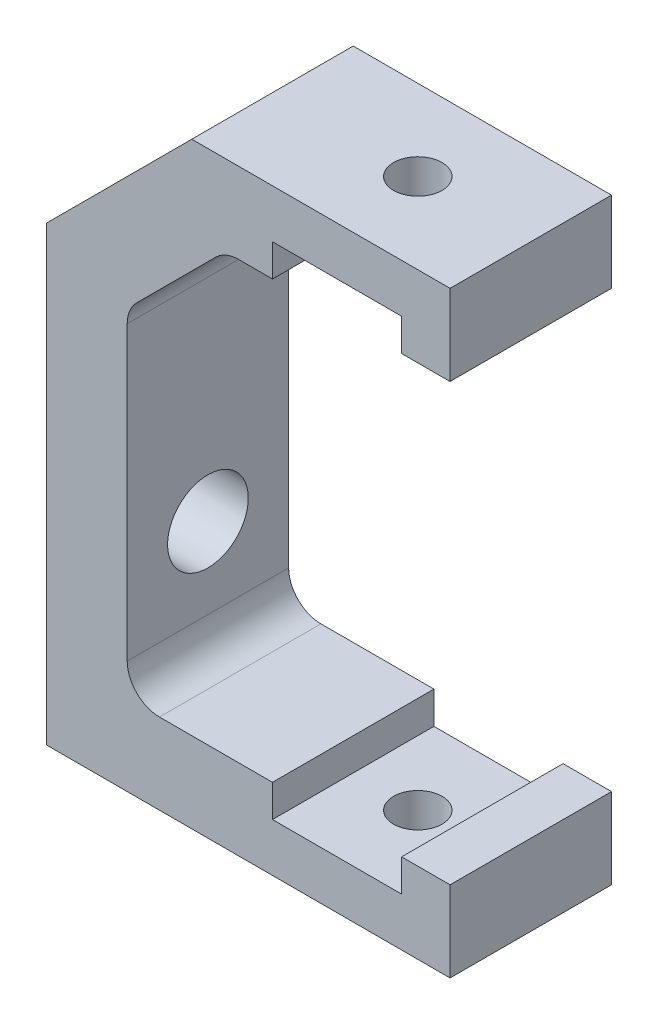
ISO-10303-21;
HEADER;
FILE_DESCRIPTION(('STEP AP214'),'2;1');
FILE_NAME('part.step','',(''),(''),'','','');
FILE_SCHEMA(('AUTOMOTIVE_DESIGN { 1 0 10303 214 1 1 1 1 }'));
ENDSEC;
DATA;
#1=APPLICATION_CONTEXT('core data for automotive mechanical design processes');
#2=APPLICATION_PROTOCOL_DEFINITION('international standard','automotive_design',2000,#1);
#3=PRODUCT_CONTEXT('',#1,'mechanical');
#4=PRODUCT('Part','Part','',(#3));
#5=PRODUCT_RELATED_PRODUCT_CATEGORY('part','',(#4));
#6=PRODUCT_DEFINITION_FORMATION('','',#4);
#7=PRODUCT_DEFINITION_CONTEXT('part definition',#1,'design');
#8=PRODUCT_DEFINITION('design','',#6,#7);
#9=PRODUCT_DEFINITION_SHAPE('','',#8);
#10=(LENGTH_UNIT() NAMED_UNIT(*) SI_UNIT(.MILLI.,.METRE.));
#11=(NAMED_UNIT(*) PLANE_ANGLE_UNIT() SI_UNIT($,.RADIAN.));
#12=(NAMED_UNIT(*) SI_UNIT($,.STERADIAN.) SOLID_ANGLE_UNIT());
#13=UNCERTAINTY_MEASURE_WITH_UNIT(LENGTH_MEASURE(1.E-05),#10,'distance_accuracy_value','');
#14=(GEOMETRIC_REPRESENTATION_CONTEXT(3) GLOBAL_UNCERTAINTY_ASSIGNED_CONTEXT((#13)) GLOBAL_UNIT_ASSIGNED_CONTEXT((#10,
#11,#12)) REPRESENTATION_CONTEXT('',''));
#15=CARTESIAN_POINT('',(0.,0.,0.));
#16=DIRECTION('',(0.,0.,1.));
#17=DIRECTION('',(1.,0.,0.));
#18=AXIS2_PLACEMENT_3D('',#15,#16,#17);
#19=CARTESIAN_POINT('',(0.,0.,10.));
#20=DIRECTION('',(0.,1.,0.));
#21=DIRECTION('',(0.,0.,1.));
#22=AXIS2_PLACEMENT_3D('',#19,#20,#21);
#23=PLANE('',#22);
#24=CARTESIAN_POINT('',(18.,0.,5.));
#25=DIRECTION('',(0.,1.,0.));
#26=DIRECTION('',(0.,0.,1.));
#27=AXIS2_PLACEMENT_3D('',#24,#25,#26);
#28=CIRCLE('',#27,1.5);
#29=CARTESIAN_POINT('',(18.,0.,6.5));
#30=VERTEX_POINT('',#29);
#31=EDGE_CURVE('E222',#30,#30,#28,.T.);
#32=ORIENTED_EDGE('',*,*,#31,.T.);
#33=EDGE_LOOP('',(#32));
#34=FACE_BOUND('',#33,.T.);
#35=DIRECTION('',(1.,0.,0.));
#36=VECTOR('',#35,1.);
#37=CARTESIAN_POINT('',(0.,0.,0.));
#38=LINE('',#37,#36);
#39=CARTESIAN_POINT('',(0.,0.,0.));
#40=VERTEX_POINT('',#39);
#41=CARTESIAN_POINT('',(25.,0.,0.));
#42=VERTEX_POINT('',#41);
#43=EDGE_CURVE('E220',#40,#42,#38,.T.);
#44=ORIENTED_EDGE('',*,*,#43,.T.);
#45=DIRECTION('',(0.,0.,-1.));
#46=VECTOR('',#45,1.);
#47=CARTESIAN_POINT('',(25.,0.,10.));
#48=LINE('',#47,#46);
#49=CARTESIAN_POINT('',(25.,0.,10.));
#50=VERTEX_POINT('',#49);
#51=EDGE_CURVE('E11',#50,#42,#48,.T.);
#52=ORIENTED_EDGE('',*,*,#51,.F.);
#53=DIRECTION('',(1.,0.,0.));
#54=VECTOR('',#53,1.);
#55=CARTESIAN_POINT('',(0.,0.,10.));
#56=LINE('',#55,#54);
#57=CARTESIAN_POINT('',(0.,0.,10.));
#58=VERTEX_POINT('',#57);
#59=EDGE_CURVE('E256',#58,#50,#56,.T.);
#60=ORIENTED_EDGE('',*,*,#59,.F.);
#61=DIRECTION('',(0.,0.,-1.));
#62=VECTOR('',#61,1.);
#63=CARTESIAN_POINT('',(0.,0.,10.));
#64=LINE('',#63,#62);
#65=EDGE_CURVE('E213',#58,#40,#64,.T.);
#66=ORIENTED_EDGE('',*,*,#65,.T.);
#67=EDGE_LOOP('',(#44,#52,#60,#66));
#68=FACE_BOUND('',#67,.T.);
#69=ADVANCED_FACE('F43',(#34,#68),#23,.F.);
#70=CARTESIAN_POINT('',(25.,0.,10.));
#71=DIRECTION('',(-1.,0.,0.));
#72=DIRECTION('',(0.,0.,1.));
#73=AXIS2_PLACEMENT_3D('',#70,#71,#72);
#74=PLANE('',#73);
#75=DIRECTION('',(0.,1.,0.));
#76=VECTOR('',#75,1.);
#77=CARTESIAN_POINT('',(25.,0.,0.));
#78=LINE('',#77,#76);
#79=CARTESIAN_POINT('',(25.,5.,0.));
#80=VERTEX_POINT('',#79);
#81=EDGE_CURVE('E219',#42,#80,#78,.T.);
#82=ORIENTED_EDGE('',*,*,#81,.T.);
#83=DIRECTION('',(0.,0.,-1.));
#84=VECTOR('',#83,1.);
#85=CARTESIAN_POINT('',(25.,5.,10.));
#86=LINE('',#85,#84);
#87=CARTESIAN_POINT('',(25.,5.,10.));
#88=VERTEX_POINT('',#87);
#89=EDGE_CURVE('E51',#88,#80,#86,.T.);
#90=ORIENTED_EDGE('',*,*,#89,.F.);
#91=DIRECTION('',(0.,1.,0.));
#92=VECTOR('',#91,1.);
#93=CARTESIAN_POINT('',(25.,0.,10.));
#94=LINE('',#93,#92);
#95=EDGE_CURVE('E143',#50,#88,#94,.T.);
#96=ORIENTED_EDGE('',*,*,#95,.F.);
#97=ORIENTED_EDGE('',*,*,#51,.T.);
#98=EDGE_LOOP('',(#82,#90,#96,#97));
#99=FACE_BOUND('',#98,.T.);
#100=ADVANCED_FACE('F382',(#99),#74,.F.);
#101=CARTESIAN_POINT('',(25.,5.,10.));
#102=DIRECTION('',(0.,-1.,0.));
#103=DIRECTION('',(0.,0.,-1.));
#104=AXIS2_PLACEMENT_3D('',#101,#102,#103);
#105=PLANE('',#104);
#106=DIRECTION('',(-1.,0.,0.));
#107=VECTOR('',#106,1.);
#108=CARTESIAN_POINT('',(25.,5.,0.));
#109=LINE('',#108,#107);
#110=CARTESIAN_POINT('',(22.,5.,0.));
#111=VERTEX_POINT('',#110);
#112=EDGE_CURVE('E224',#80,#111,#109,.T.);
#113=ORIENTED_EDGE('',*,*,#112,.T.);
#114=DIRECTION('',(0.,0.,-1.));
#115=VECTOR('',#114,1.);
#116=CARTESIAN_POINT('',(22.,5.,10.));
#117=LINE('',#116,#115);
#118=CARTESIAN_POINT('',(22.,5.,10.));
#119=VERTEX_POINT('',#118);
#120=EDGE_CURVE('E301',#119,#111,#117,.T.);
#121=ORIENTED_EDGE('',*,*,#120,.F.);
#122=DIRECTION('',(-1.,0.,0.));
#123=VECTOR('',#122,1.);
#124=CARTESIAN_POINT('',(25.,5.,10.));
#125=LINE('',#124,#123);
#126=EDGE_CURVE('E315',#88,#119,#125,.T.);
#127=ORIENTED_EDGE('',*,*,#126,.F.);
#128=ORIENTED_EDGE('',*,*,#89,.T.);
#129=EDGE_LOOP('',(#113,#121,#127,#128));
#130=FACE_BOUND('',#129,.T.);
#131=ADVANCED_FACE('F309',(#130),#105,.F.);
#132=CARTESIAN_POINT('',(22.,5.,10.));
#133=DIRECTION('',(1.,0.,0.));
#134=DIRECTION('',(0.,0.,-1.));
#135=AXIS2_PLACEMENT_3D('',#132,#133,#134);
#136=PLANE('',#135);
#137=DIRECTION('',(0.,-1.,0.));
#138=VECTOR('',#137,1.);
#139=CARTESIAN_POINT('',(22.,5.,0.));
#140=LINE('',#139,#138);
#141=CARTESIAN_POINT('',(22.,3.,0.));
#142=VERTEX_POINT('',#141);
#143=EDGE_CURVE('E223',#111,#142,#140,.T.);
#144=ORIENTED_EDGE('',*,*,#143,.T.);
#145=DIRECTION('',(0.,0.,-1.));
#146=VECTOR('',#145,1.);
#147=CARTESIAN_POINT('',(22.,3.,10.));
#148=LINE('',#147,#146);
#149=CARTESIAN_POINT('',(22.,3.,10.));
#150=VERTEX_POINT('',#149);
#151=EDGE_CURVE('E302',#150,#142,#148,.T.);
#152=ORIENTED_EDGE('',*,*,#151,.F.);
#153=DIRECTION('',(0.,-1.,0.));
#154=VECTOR('',#153,1.);
#155=CARTESIAN_POINT('',(22.,5.,10.));
#156=LINE('',#155,#154);
#157=EDGE_CURVE('E329',#119,#150,#156,.T.);
#158=ORIENTED_EDGE('',*,*,#157,.F.);
#159=ORIENTED_EDGE('',*,*,#120,.T.);
#160=EDGE_LOOP('',(#144,#152,#158,#159));
#161=FACE_BOUND('',#160,.T.);
#162=ADVANCED_FACE('F321',(#161),#136,.F.);
#163=CARTESIAN_POINT('',(22.,3.,10.));
#164=DIRECTION('',(0.,-1.,0.));
#165=DIRECTION('',(0.,0.,-1.));
#166=AXIS2_PLACEMENT_3D('',#163,#164,#165);
#167=PLANE('',#166);
#168=CARTESIAN_POINT('',(18.,3.,5.));
#169=DIRECTION('',(0.,1.,0.));
#170=DIRECTION('',(0.,0.,1.));
#171=AXIS2_PLACEMENT_3D('',#168,#169,#170);
#172=CIRCLE('',#171,1.5);
#173=CARTESIAN_POINT('',(18.,3.,6.5));
#174=VERTEX_POINT('',#173);
#175=EDGE_CURVE('E391',#174,#174,#172,.T.);
#176=ORIENTED_EDGE('',*,*,#175,.F.);
#177=EDGE_LOOP('',(#176));
#178=FACE_BOUND('',#177,.T.);
#179=DIRECTION('',(-1.,0.,0.));
#180=VECTOR('',#179,1.);
#181=CARTESIAN_POINT('',(22.,3.,0.));
#182=LINE('',#181,#180);
#183=CARTESIAN_POINT('',(14.,3.,0.));
#184=VERTEX_POINT('',#183);
#185=EDGE_CURVE('E227',#142,#184,#182,.T.);
#186=ORIENTED_EDGE('',*,*,#185,.T.);
#187=DIRECTION('',(0.,0.,-1.));
#188=VECTOR('',#187,1.);
#189=CARTESIAN_POINT('',(14.,3.,10.));
#190=LINE('',#189,#188);
#191=CARTESIAN_POINT('',(14.,3.,10.));
#192=VERTEX_POINT('',#191);
#193=EDGE_CURVE('E299',#192,#184,#190,.T.);
#194=ORIENTED_EDGE('',*,*,#193,.F.);
#195=DIRECTION('',(-1.,0.,0.));
#196=VECTOR('',#195,1.);
#197=CARTESIAN_POINT('',(22.,3.,10.));
#198=LINE('',#197,#196);
#199=EDGE_CURVE('E330',#150,#192,#198,.T.);
#200=ORIENTED_EDGE('',*,*,#199,.F.);
#201=ORIENTED_EDGE('',*,*,#151,.T.);
#202=EDGE_LOOP('',(#186,#194,#200,#201));
#203=FACE_BOUND('',#202,.T.);
#204=ADVANCED_FACE('F324',(#178,#203),#167,.F.);
#205=CARTESIAN_POINT('',(14.,3.,10.));
#206=DIRECTION('',(-1.,0.,0.));
#207=DIRECTION('',(0.,0.,1.));
#208=AXIS2_PLACEMENT_3D('',#205,#206,#207);
#209=PLANE('',#208);
#210=DIRECTION('',(0.,1.,0.));
#211=VECTOR('',#210,1.);
#212=CARTESIAN_POINT('',(14.,3.,0.));
#213=LINE('',#212,#211);
#214=CARTESIAN_POINT('',(14.,5.,0.));
#215=VERTEX_POINT('',#214);
#216=EDGE_CURVE('E228',#184,#215,#213,.T.);
#217=ORIENTED_EDGE('',*,*,#216,.T.);
#218=DIRECTION('',(0.,0.,-1.));
#219=VECTOR('',#218,1.);
#220=CARTESIAN_POINT('',(14.,5.,10.));
#221=LINE('',#220,#219);
#222=CARTESIAN_POINT('',(14.,5.,10.));
#223=VERTEX_POINT('',#222);
#224=EDGE_CURVE('E293',#223,#215,#221,.T.);
#225=ORIENTED_EDGE('',*,*,#224,.F.);
#226=DIRECTION('',(0.,1.,0.));
#227=VECTOR('',#226,1.);
#228=CARTESIAN_POINT('',(14.,3.,10.));
#229=LINE('',#228,#227);
#230=EDGE_CURVE('E328',#192,#223,#229,.T.);
#231=ORIENTED_EDGE('',*,*,#230,.F.);
#232=ORIENTED_EDGE('',*,*,#193,.T.);
#233=EDGE_LOOP('',(#217,#225,#231,#232));
#234=FACE_BOUND('',#233,.T.);
#235=ADVANCED_FACE('F451',(#234),#209,.F.);
#236=CARTESIAN_POINT('',(7.00000000000002,5.,10.));
#237=DIRECTION('',(0.,-1.,0.));
#238=DIRECTION('',(0.,0.,-1.));
#239=AXIS2_PLACEMENT_3D('',#236,#237,#238);
#240=PLANE('',#239);
#241=DIRECTION('',(-1.,0.,0.));
#242=VECTOR('',#241,1.);
#243=CARTESIAN_POINT('',(7.00000000000002,5.,0.));
#244=LINE('',#243,#242);
#245=CARTESIAN_POINT('',(7.00000000000002,5.,0.));
#246=VERTEX_POINT('',#245);
#247=EDGE_CURVE('E232',#215,#246,#244,.T.);
#248=ORIENTED_EDGE('',*,*,#247,.T.);
#249=DIRECTION('',(0.,0.,-1.));
#250=VECTOR('',#249,1.);
#251=CARTESIAN_POINT('',(7.00000000000002,5.,10.));
#252=LINE('',#251,#250);
#253=CARTESIAN_POINT('',(7.00000000000002,5.,10.));
#254=VERTEX_POINT('',#253);
#255=EDGE_CURVE('E295',#254,#246,#252,.T.);
#256=ORIENTED_EDGE('',*,*,#255,.F.);
#257=DIRECTION('',(-1.,0.,0.));
#258=VECTOR('',#257,1.);
#259=CARTESIAN_POINT('',(7.00000000000002,5.,10.));
#260=LINE('',#259,#258);
#261=EDGE_CURVE('E335',#223,#254,#260,.T.);
#262=ORIENTED_EDGE('',*,*,#261,.F.);
#263=ORIENTED_EDGE('',*,*,#224,.T.);
#264=EDGE_LOOP('',(#248,#256,#262,#263));
#265=FACE_BOUND('',#264,.T.);
#266=ADVANCED_FACE('F452',(#265),#240,.F.);
#267=CARTESIAN_POINT('',(7.,7.,10.));
#268=DIRECTION('',(0.,0.,-1.));
#269=DIRECTION('',(-1.,0.,0.));
#270=AXIS2_PLACEMENT_3D('',#267,#268,#269);
#271=CYLINDRICAL_SURFACE('',#270,2.);
#272=CARTESIAN_POINT('',(7.,7.,0.));
#273=DIRECTION('',(0.,0.,-1.));
#274=DIRECTION('',(-1.,0.,0.));
#275=AXIS2_PLACEMENT_3D('',#272,#273,#274);
#276=CIRCLE('',#275,2.);
#277=CARTESIAN_POINT('',(5.,7.00000000000002,0.));
#278=VERTEX_POINT('',#277);
#279=EDGE_CURVE('E234',#246,#278,#276,.T.);
#280=ORIENTED_EDGE('',*,*,#279,.T.);
#281=DIRECTION('',(0.,0.,-1.));
#282=VECTOR('',#281,1.);
#283=CARTESIAN_POINT('',(5.,7.00000000000002,10.));
#284=LINE('',#283,#282);
#285=CARTESIAN_POINT('',(5.,7.00000000000002,10.));
#286=VERTEX_POINT('',#285);
#287=EDGE_CURVE('E286',#286,#278,#284,.T.);
#288=ORIENTED_EDGE('',*,*,#287,.F.);
#289=CARTESIAN_POINT('',(7.,7.,10.));
#290=DIRECTION('',(0.,0.,-1.));
#291=DIRECTION('',(-1.,0.,0.));
#292=AXIS2_PLACEMENT_3D('',#289,#290,#291);
#293=CIRCLE('',#292,2.);
#294=EDGE_CURVE('E339',#254,#286,#293,.T.);
#295=ORIENTED_EDGE('',*,*,#294,.F.);
#296=ORIENTED_EDGE('',*,*,#255,.T.);
#297=EDGE_LOOP('',(#280,#288,#295,#296));
#298=FACE_BOUND('',#297,.T.);
#299=ADVANCED_FACE('F423',(#298),#271,.F.);
#300=CARTESIAN_POINT('',(5.,25.1005050633883,10.));
#301=DIRECTION('',(-1.,0.,0.));
#302=DIRECTION('',(0.,-1.,0.));
#303=AXIS2_PLACEMENT_3D('',#300,#301,#302);
#304=PLANE('',#303);
#305=CARTESIAN_POINT('',(5.,12.,5.));
#306=DIRECTION('',(-1.,0.,0.));
#307=DIRECTION('',(0.,-1.,0.));
#308=AXIS2_PLACEMENT_3D('',#305,#306,#307);
#309=CIRCLE('',#308,2.5);
#310=CARTESIAN_POINT('',(5.,9.5,5.));
#311=VERTEX_POINT('',#310);
#312=EDGE_CURVE('E404',#311,#311,#309,.T.);
#313=ORIENTED_EDGE('',*,*,#312,.T.);
#314=EDGE_LOOP('',(#313));
#315=FACE_BOUND('',#314,.T.);
#316=DIRECTION('',(0.,1.,0.));
#317=VECTOR('',#316,1.);
#318=CARTESIAN_POINT('',(5.,25.1005050633883,0.));
#319=LINE('',#318,#317);
#320=CARTESIAN_POINT('',(5.,25.1005050633883,0.));
#321=VERTEX_POINT('',#320);
#322=EDGE_CURVE('E233',#278,#321,#319,.T.);
#323=ORIENTED_EDGE('',*,*,#322,.T.);
#324=DIRECTION('',(0.,0.,-1.));
#325=VECTOR('',#324,1.);
#326=CARTESIAN_POINT('',(5.,25.1005050633883,10.));
#327=LINE('',#326,#325);
#328=CARTESIAN_POINT('',(5.,25.1005050633883,10.));
#329=VERTEX_POINT('',#328);
#330=EDGE_CURVE('E287',#329,#321,#327,.T.);
#331=ORIENTED_EDGE('',*,*,#330,.F.);
#332=DIRECTION('',(0.,1.,0.));
#333=VECTOR('',#332,1.);
#334=CARTESIAN_POINT('',(5.,25.1005050633883,10.));
#335=LINE('',#334,#333);
#336=EDGE_CURVE('E340',#286,#329,#335,.T.);
#337=ORIENTED_EDGE('',*,*,#336,.F.);
#338=ORIENTED_EDGE('',*,*,#287,.T.);
#339=EDGE_LOOP('',(#323,#331,#337,#338));
#340=FACE_BOUND('',#339,.T.);
#341=ADVANCED_FACE('F417',(#315,#340),#304,.F.);
#342=CARTESIAN_POINT('',(7.,25.1005050633883,10.));
#343=DIRECTION('',(0.,0.,-1.));
#344=DIRECTION('',(-1.,0.,0.));
#345=AXIS2_PLACEMENT_3D('',#342,#343,#344);
#346=CYLINDRICAL_SURFACE('',#345,2.);
#347=CARTESIAN_POINT('',(7.,25.1005050633883,0.));
#348=DIRECTION('',(0.,0.,-1.));
#349=DIRECTION('',(1.,0.,0.));
#350=AXIS2_PLACEMENT_3D('',#347,#348,#349);
#351=CIRCLE('',#350,2.);
#352=CARTESIAN_POINT('',(5.5857864376269,26.5147186257614,0.));
#353=VERTEX_POINT('',#352);
#354=EDGE_CURVE('E240',#321,#353,#351,.T.);
#355=ORIENTED_EDGE('',*,*,#354,.T.);
#356=DIRECTION('',(0.,0.,-1.));
#357=VECTOR('',#356,1.);
#358=CARTESIAN_POINT('',(5.5857864376269,26.5147186257614,10.));
#359=LINE('',#358,#357);
#360=CARTESIAN_POINT('',(5.5857864376269,26.5147186257614,10.));
#361=VERTEX_POINT('',#360);
#362=EDGE_CURVE('E284',#361,#353,#359,.T.);
#363=ORIENTED_EDGE('',*,*,#362,.F.);
#364=CARTESIAN_POINT('',(7.,25.1005050633883,10.));
#365=DIRECTION('',(0.,0.,-1.));
#366=DIRECTION('',(1.,0.,0.));
#367=AXIS2_PLACEMENT_3D('',#364,#365,#366);
#368=CIRCLE('',#367,2.);
#369=EDGE_CURVE('E345',#329,#361,#368,.T.);
#370=ORIENTED_EDGE('',*,*,#369,.F.);
#371=ORIENTED_EDGE('',*,*,#330,.T.);
#372=EDGE_LOOP('',(#355,#363,#370,#371));
#373=FACE_BOUND('',#372,.T.);
#374=ADVANCED_FACE('F419',(#373),#346,.F.);
#375=CARTESIAN_POINT('',(5.5857864376269,26.5147186257614,10.));
#376=DIRECTION('',(-0.707106781186549,0.707106781186546,0.));
#377=DIRECTION('',(-0.707106781186546,-0.707106781186549,0.));
#378=AXIS2_PLACEMENT_3D('',#375,#376,#377);
#379=PLANE('',#378);
#380=DIRECTION('',(0.707106781186546,0.707106781186549,0.));
#381=VECTOR('',#380,1.);
#382=CARTESIAN_POINT('',(5.5857864376269,26.5147186257614,0.));
#383=LINE('',#382,#381);
#384=CARTESIAN_POINT('',(10.4852813742385,31.4142135623731,0.));
#385=VERTEX_POINT('',#384);
#386=EDGE_CURVE('E239',#353,#385,#383,.T.);
#387=ORIENTED_EDGE('',*,*,#386,.T.);
#388=DIRECTION('',(0.,0.,-1.));
#389=VECTOR('',#388,1.);
#390=CARTESIAN_POINT('',(10.4852813742385,31.4142135623731,10.));
#391=LINE('',#390,#389);
#392=CARTESIAN_POINT('',(10.4852813742385,31.4142135623731,10.));
#393=VERTEX_POINT('',#392);
#394=EDGE_CURVE('E278',#393,#385,#391,.T.);
#395=ORIENTED_EDGE('',*,*,#394,.F.);
#396=DIRECTION('',(0.707106781186546,0.707106781186549,0.));
#397=VECTOR('',#396,1.);
#398=CARTESIAN_POINT('',(5.5857864376269,26.5147186257614,10.));
#399=LINE('',#398,#397);
#400=EDGE_CURVE('E341',#361,#393,#399,.T.);
#401=ORIENTED_EDGE('',*,*,#400,.F.);
#402=ORIENTED_EDGE('',*,*,#362,.T.);
#403=EDGE_LOOP('',(#387,#395,#401,#402));
#404=FACE_BOUND('',#403,.T.);
#405=ADVANCED_FACE('F440',(#404),#379,.F.);
#406=CARTESIAN_POINT('',(11.8994949366116,30.,10.));
#407=DIRECTION('',(0.,0.,-1.));
#408=DIRECTION('',(-1.,0.,0.));
#409=AXIS2_PLACEMENT_3D('',#406,#407,#408);
#410=CYLINDRICAL_SURFACE('',#409,2.);
#411=CARTESIAN_POINT('',(11.8994949366116,30.,0.));
#412=DIRECTION('',(0.,0.,-1.));
#413=DIRECTION('',(1.,0.,0.));
#414=AXIS2_PLACEMENT_3D('',#411,#412,#413);
#415=CIRCLE('',#414,2.);
#416=CARTESIAN_POINT('',(11.8994949366116,32.,0.));
#417=VERTEX_POINT('',#416);
#418=EDGE_CURVE('E241',#385,#417,#415,.T.);
#419=ORIENTED_EDGE('',*,*,#418,.T.);
#420=DIRECTION('',(0.,0.,-1.));
#421=VECTOR('',#420,1.);
#422=CARTESIAN_POINT('',(11.8994949366116,32.,10.));
#423=LINE('',#422,#421);
#424=CARTESIAN_POINT('',(11.8994949366116,32.,10.));
#425=VERTEX_POINT('',#424);
#426=EDGE_CURVE('E280',#425,#417,#423,.T.);
#427=ORIENTED_EDGE('',*,*,#426,.F.);
#428=CARTESIAN_POINT('',(11.8994949366116,30.,10.));
#429=DIRECTION('',(0.,0.,-1.));
#430=DIRECTION('',(1.,0.,0.));
#431=AXIS2_PLACEMENT_3D('',#428,#429,#430);
#432=CIRCLE('',#431,2.);
#433=EDGE_CURVE('E347',#393,#425,#432,.T.);
#434=ORIENTED_EDGE('',*,*,#433,.F.);
#435=ORIENTED_EDGE('',*,*,#394,.T.);
#436=EDGE_LOOP('',(#419,#427,#434,#435));
#437=FACE_BOUND('',#436,.T.);
#438=ADVANCED_FACE('F442',(#437),#410,.F.);
#439=CARTESIAN_POINT('',(11.8994949366116,32.,10.));
#440=DIRECTION('',(0.,1.,0.));
#441=DIRECTION('',(0.,0.,1.));
#442=AXIS2_PLACEMENT_3D('',#439,#440,#441);
#443=PLANE('',#442);
#444=DIRECTION('',(1.,0.,0.));
#445=VECTOR('',#444,1.);
#446=CARTESIAN_POINT('',(11.8994949366116,32.,0.));
#447=LINE('',#446,#445);
#448=CARTESIAN_POINT('',(14.,32.,0.));
#449=VERTEX_POINT('',#448);
#450=EDGE_CURVE('E244',#417,#449,#447,.T.);
#451=ORIENTED_EDGE('',*,*,#450,.T.);
#452=DIRECTION('',(0.,0.,-1.));
#453=VECTOR('',#452,1.);
#454=CARTESIAN_POINT('',(14.,32.,10.));
#455=LINE('',#454,#453);
#456=CARTESIAN_POINT('',(14.,32.,10.));
#457=VERTEX_POINT('',#456);
#458=EDGE_CURVE('E273',#457,#449,#455,.T.);
#459=ORIENTED_EDGE('',*,*,#458,.F.);
#460=DIRECTION('',(1.,0.,0.));
#461=VECTOR('',#460,1.);
#462=CARTESIAN_POINT('',(11.8994949366116,32.,10.));
#463=LINE('',#462,#461);
#464=EDGE_CURVE('E346',#425,#457,#463,.T.);
#465=ORIENTED_EDGE('',*,*,#464,.F.);
#466=ORIENTED_EDGE('',*,*,#426,.T.);
#467=EDGE_LOOP('',(#451,#459,#465,#466));
#468=FACE_BOUND('',#467,.T.);
#469=ADVANCED_FACE('F531',(#468),#443,.F.);
#470=CARTESIAN_POINT('',(14.,34.,10.));
#471=DIRECTION('',(-1.,0.,0.));
#472=DIRECTION('',(0.,0.,1.));
#473=AXIS2_PLACEMENT_3D('',#470,#471,#472);
#474=PLANE('',#473);
#475=DIRECTION('',(0.,1.,0.));
#476=VECTOR('',#475,1.);
#477=CARTESIAN_POINT('',(14.,34.,0.));
#478=LINE('',#477,#476);
#479=CARTESIAN_POINT('',(14.,34.,0.));
#480=VERTEX_POINT('',#479);
#481=EDGE_CURVE('E245',#449,#480,#478,.T.);
#482=ORIENTED_EDGE('',*,*,#481,.T.);
#483=DIRECTION('',(0.,0.,-1.));
#484=VECTOR('',#483,1.);
#485=CARTESIAN_POINT('',(14.,34.,10.));
#486=LINE('',#485,#484);
#487=CARTESIAN_POINT('',(14.,34.,10.));
#488=VERTEX_POINT('',#487);
#489=EDGE_CURVE('E271',#488,#480,#486,.T.);
#490=ORIENTED_EDGE('',*,*,#489,.F.);
#491=DIRECTION('',(0.,1.,0.));
#492=VECTOR('',#491,1.);
#493=CARTESIAN_POINT('',(14.,34.,10.));
#494=LINE('',#493,#492);
#495=EDGE_CURVE('E348',#457,#488,#494,.T.);
#496=ORIENTED_EDGE('',*,*,#495,.F.);
#497=ORIENTED_EDGE('',*,*,#458,.T.);
#498=EDGE_LOOP('',(#482,#490,#496,#497));
#499=FACE_BOUND('',#498,.T.);
#500=ADVANCED_FACE('F545',(#499),#474,.F.);
#501=CARTESIAN_POINT('',(22.,34.,10.));
#502=DIRECTION('',(0.,1.,0.));
#503=DIRECTION('',(0.,0.,1.));
#504=AXIS2_PLACEMENT_3D('',#501,#502,#503);
#505=PLANE('',#504);
#506=CARTESIAN_POINT('',(18.,34.,5.));
#507=DIRECTION('',(0.,1.,0.));
#508=DIRECTION('',(0.,0.,1.));
#509=AXIS2_PLACEMENT_3D('',#506,#507,#508);
#510=CIRCLE('',#509,1.5);
#511=CARTESIAN_POINT('',(18.,34.,6.5));
#512=VERTEX_POINT('',#511);
#513=EDGE_CURVE('E393',#512,#512,#510,.T.);
#514=ORIENTED_EDGE('',*,*,#513,.T.);
#515=EDGE_LOOP('',(#514));
#516=FACE_BOUND('',#515,.T.);
#517=DIRECTION('',(1.,0.,0.));
#518=VECTOR('',#517,1.);
#519=CARTESIAN_POINT('',(22.,34.,0.));
#520=LINE('',#519,#518);
#521=CARTESIAN_POINT('',(22.,34.,0.));
#522=VERTEX_POINT('',#521);
#523=EDGE_CURVE('E250',#480,#522,#520,.T.);
#524=ORIENTED_EDGE('',*,*,#523,.T.);
#525=DIRECTION('',(0.,0.,-1.));
#526=VECTOR('',#525,1.);
#527=CARTESIAN_POINT('',(22.,34.,10.));
#528=LINE('',#527,#526);
#529=CARTESIAN_POINT('',(22.,34.,10.));
#530=VERTEX_POINT('',#529);
#531=EDGE_CURVE('E268',#530,#522,#528,.T.);
#532=ORIENTED_EDGE('',*,*,#531,.F.);
#533=DIRECTION('',(1.,0.,0.));
#534=VECTOR('',#533,1.);
#535=CARTESIAN_POINT('',(22.,34.,10.));
#536=LINE('',#535,#534);
#537=EDGE_CURVE('E352',#488,#530,#536,.T.);
#538=ORIENTED_EDGE('',*,*,#537,.F.);
#539=ORIENTED_EDGE('',*,*,#489,.T.);
#540=EDGE_LOOP('',(#524,#532,#538,#539));
#541=FACE_BOUND('',#540,.T.);
#542=ADVANCED_FACE('F555',(#516,#541),#505,.F.);
#543=CARTESIAN_POINT('',(22.,32.,10.));
#544=DIRECTION('',(1.,0.,0.));
#545=DIRECTION('',(0.,0.,-1.));
#546=AXIS2_PLACEMENT_3D('',#543,#544,#545);
#547=PLANE('',#546);
#548=DIRECTION('',(0.,-1.,0.));
#549=VECTOR('',#548,1.);
#550=CARTESIAN_POINT('',(22.,32.,0.));
#551=LINE('',#550,#549);
#552=CARTESIAN_POINT('',(22.,32.,0.));
#553=VERTEX_POINT('',#552);
#554=EDGE_CURVE('E246',#522,#553,#551,.T.);
#555=ORIENTED_EDGE('',*,*,#554,.T.);
#556=DIRECTION('',(0.,0.,-1.));
#557=VECTOR('',#556,1.);
#558=CARTESIAN_POINT('',(22.,32.,10.));
#559=LINE('',#558,#557);
#560=CARTESIAN_POINT('',(22.,32.,10.));
#561=VERTEX_POINT('',#560);
#562=EDGE_CURVE('E264',#561,#553,#559,.T.);
#563=ORIENTED_EDGE('',*,*,#562,.F.);
#564=DIRECTION('',(0.,-1.,0.));
#565=VECTOR('',#564,1.);
#566=CARTESIAN_POINT('',(22.,32.,10.));
#567=LINE('',#566,#565);
#568=EDGE_CURVE('E353',#530,#561,#567,.T.);
#569=ORIENTED_EDGE('',*,*,#568,.F.);
#570=ORIENTED_EDGE('',*,*,#531,.T.);
#571=EDGE_LOOP('',(#555,#563,#569,#570));
#572=FACE_BOUND('',#571,.T.);
#573=ADVANCED_FACE('F564',(#572),#547,.F.);
#574=CARTESIAN_POINT('',(25.,32.,10.));
#575=DIRECTION('',(0.,1.,0.));
#576=DIRECTION('',(0.,0.,1.));
#577=AXIS2_PLACEMENT_3D('',#574,#575,#576);
#578=PLANE('',#577);
#579=DIRECTION('',(1.,0.,0.));
#580=VECTOR('',#579,1.);
#581=CARTESIAN_POINT('',(25.,32.,0.));
#582=LINE('',#581,#580);
#583=CARTESIAN_POINT('',(25.,32.,0.));
#584=VERTEX_POINT('',#583);
#585=EDGE_CURVE('E253',#553,#584,#582,.T.);
#586=ORIENTED_EDGE('',*,*,#585,.T.);
#587=DIRECTION('',(0.,0.,-1.));
#588=VECTOR('',#587,1.);
#589=CARTESIAN_POINT('',(25.,32.,10.));
#590=LINE('',#589,#588);
#591=CARTESIAN_POINT('',(25.,32.,10.));
#592=VERTEX_POINT('',#591);
#593=EDGE_CURVE('E265',#592,#584,#590,.T.);
#594=ORIENTED_EDGE('',*,*,#593,.F.);
#595=DIRECTION('',(1.,0.,0.));
#596=VECTOR('',#595,1.);
#597=CARTESIAN_POINT('',(25.,32.,10.));
#598=LINE('',#597,#596);
#599=EDGE_CURVE('E357',#561,#592,#598,.T.);
#600=ORIENTED_EDGE('',*,*,#599,.F.);
#601=ORIENTED_EDGE('',*,*,#562,.T.);
#602=EDGE_LOOP('',(#586,#594,#600,#601));
#603=FACE_BOUND('',#602,.T.);
#604=ADVANCED_FACE('F362',(#603),#578,.F.);
#605=CARTESIAN_POINT('',(25.,37.,10.));
#606=DIRECTION('',(-1.,0.,0.));
#607=DIRECTION('',(0.,0.,1.));
#608=AXIS2_PLACEMENT_3D('',#605,#606,#607);
#609=PLANE('',#608);
#610=DIRECTION('',(0.,1.,0.));
#611=VECTOR('',#610,1.);
#612=CARTESIAN_POINT('',(25.,37.,0.));
#613=LINE('',#612,#611);
#614=CARTESIAN_POINT('',(25.,37.,0.));
#615=VERTEX_POINT('',#614);
#616=EDGE_CURVE('E251',#584,#615,#613,.T.);
#617=ORIENTED_EDGE('',*,*,#616,.T.);
#618=DIRECTION('',(0.,0.,-1.));
#619=VECTOR('',#618,1.);
#620=CARTESIAN_POINT('',(25.,37.,10.));
#621=LINE('',#620,#619);
#622=CARTESIAN_POINT('',(25.,37.,10.));
#623=VERTEX_POINT('',#622);
#624=EDGE_CURVE('E208',#623,#615,#621,.T.);
#625=ORIENTED_EDGE('',*,*,#624,.F.);
#626=DIRECTION('',(0.,1.,0.));
#627=VECTOR('',#626,1.);
#628=CARTESIAN_POINT('',(25.,37.,10.));
#629=LINE('',#628,#627);
#630=EDGE_CURVE('E200',#592,#623,#629,.T.);
#631=ORIENTED_EDGE('',*,*,#630,.F.);
#632=ORIENTED_EDGE('',*,*,#593,.T.);
#633=EDGE_LOOP('',(#617,#625,#631,#632));
#634=FACE_BOUND('',#633,.T.);
#635=ADVANCED_FACE('F368',(#634),#609,.F.);
#636=CARTESIAN_POINT('',(25.,37.,10.));
#637=DIRECTION('',(0.,-1.,0.));
#638=DIRECTION('',(0.,0.,-1.));
#639=AXIS2_PLACEMENT_3D('',#636,#637,#638);
#640=PLANE('',#639);
#641=CARTESIAN_POINT('',(18.,37.,5.));
#642=DIRECTION('',(0.,1.,0.));
#643=DIRECTION('',(0.,0.,1.));
#644=AXIS2_PLACEMENT_3D('',#641,#642,#643);
#645=CIRCLE('',#644,1.5);
#646=CARTESIAN_POINT('',(18.,37.,6.5));
#647=VERTEX_POINT('',#646);
#648=EDGE_CURVE('E402',#647,#647,#645,.T.);
#649=ORIENTED_EDGE('',*,*,#648,.F.);
#650=EDGE_LOOP('',(#649));
#651=FACE_BOUND('',#650,.T.);
#652=DIRECTION('',(-1.,0.,0.));
#653=VECTOR('',#652,1.);
#654=CARTESIAN_POINT('',(25.,37.,0.));
#655=LINE('',#654,#653);
#656=CARTESIAN_POINT('',(8.99999999999996,37.,0.));
#657=VERTEX_POINT('',#656);
#658=EDGE_CURVE('E210',#615,#657,#655,.T.);
#659=ORIENTED_EDGE('',*,*,#658,.T.);
#660=DIRECTION('',(0.,0.,-1.));
#661=VECTOR('',#660,1.);
#662=CARTESIAN_POINT('',(8.99999999999996,37.,10.));
#663=LINE('',#662,#661);
#664=CARTESIAN_POINT('',(8.99999999999996,37.,10.));
#665=VERTEX_POINT('',#664);
#666=EDGE_CURVE('E204',#665,#657,#663,.T.);
#667=ORIENTED_EDGE('',*,*,#666,.F.);
#668=DIRECTION('',(-1.,0.,0.));
#669=VECTOR('',#668,1.);
#670=CARTESIAN_POINT('',(25.,37.,10.));
#671=LINE('',#670,#669);
#672=EDGE_CURVE('E194',#623,#665,#671,.T.);
#673=ORIENTED_EDGE('',*,*,#672,.F.);
#674=ORIENTED_EDGE('',*,*,#624,.T.);
#675=EDGE_LOOP('',(#659,#667,#673,#674));
#676=FACE_BOUND('',#675,.T.);
#677=ADVANCED_FACE('F202',(#651,#676),#640,.F.);
#678=CARTESIAN_POINT('',(0.,28.,10.));
#679=DIRECTION('',(0.707106781186549,-0.707106781186546,0.));
#680=DIRECTION('',(0.707106781186546,0.707106781186549,0.));
#681=AXIS2_PLACEMENT_3D('',#678,#679,#680);
#682=PLANE('',#681);
#683=DIRECTION('',(-0.707106781186546,-0.707106781186549,0.));
#684=VECTOR('',#683,1.);
#685=CARTESIAN_POINT('',(0.,28.,0.));
#686=LINE('',#685,#684);
#687=CARTESIAN_POINT('',(0.,28.,0.));
#688=VERTEX_POINT('',#687);
#689=EDGE_CURVE('E130',#657,#688,#686,.T.);
#690=ORIENTED_EDGE('',*,*,#689,.T.);
#691=DIRECTION('',(0.,0.,-1.));
#692=VECTOR('',#691,1.);
#693=CARTESIAN_POINT('',(0.,28.,10.));
#694=LINE('',#693,#692);
#695=CARTESIAN_POINT('',(0.,28.,10.));
#696=VERTEX_POINT('',#695);
#697=EDGE_CURVE('E207',#696,#688,#694,.T.);
#698=ORIENTED_EDGE('',*,*,#697,.F.);
#699=DIRECTION('',(-0.707106781186546,-0.707106781186549,0.));
#700=VECTOR('',#699,1.);
#701=CARTESIAN_POINT('',(0.,28.,10.));
#702=LINE('',#701,#700);
#703=EDGE_CURVE('E197',#665,#696,#702,.T.);
#704=ORIENTED_EDGE('',*,*,#703,.F.);
#705=ORIENTED_EDGE('',*,*,#666,.T.);
#706=EDGE_LOOP('',(#690,#698,#704,#705));
#707=FACE_BOUND('',#706,.T.);
#708=ADVANCED_FACE('F211',(#707),#682,.F.);
#709=CARTESIAN_POINT('',(0.,0.,10.));
#710=DIRECTION('',(1.,0.,0.));
#711=DIRECTION('',(0.,0.,-1.));
#712=AXIS2_PLACEMENT_3D('',#709,#710,#711);
#713=PLANE('',#712);
#714=CARTESIAN_POINT('',(0.,12.,5.));
#715=DIRECTION('',(-1.,0.,0.));
#716=DIRECTION('',(0.,0.,1.));
#717=AXIS2_PLACEMENT_3D('',#714,#715,#716);
#718=CIRCLE('',#717,2.5);
#719=CARTESIAN_POINT('',(0.,12.,7.5));
#720=VERTEX_POINT('',#719);
#721=EDGE_CURVE('E407',#720,#720,#718,.T.);
#722=ORIENTED_EDGE('',*,*,#721,.F.);
#723=EDGE_LOOP('',(#722));
#724=FACE_BOUND('',#723,.T.);
#725=DIRECTION('',(0.,-1.,0.));
#726=VECTOR('',#725,1.);
#727=CARTESIAN_POINT('',(0.,0.,0.));
#728=LINE('',#727,#726);
#729=EDGE_CURVE('E134',#688,#40,#728,.T.);
#730=ORIENTED_EDGE('',*,*,#729,.T.);
#731=ORIENTED_EDGE('',*,*,#65,.F.);
#732=DIRECTION('',(0.,-1.,0.));
#733=VECTOR('',#732,1.);
#734=CARTESIAN_POINT('',(0.,0.,10.));
#735=LINE('',#734,#733);
#736=EDGE_CURVE('E56',#696,#58,#735,.T.);
#737=ORIENTED_EDGE('',*,*,#736,.F.);
#738=ORIENTED_EDGE('',*,*,#697,.T.);
#739=EDGE_LOOP('',(#730,#731,#737,#738));
#740=FACE_BOUND('',#739,.T.);
#741=ADVANCED_FACE('F367',(#724,#740),#713,.F.);
#742=CARTESIAN_POINT('',(7.,7.,10.));
#743=DIRECTION('',(0.,0.,-1.));
#744=DIRECTION('',(-1.,0.,0.));
#745=AXIS2_PLACEMENT_3D('',#742,#743,#744);
#746=PLANE('',#745);
#747=ORIENTED_EDGE('',*,*,#59,.T.);
#748=ORIENTED_EDGE('',*,*,#95,.T.);
#749=ORIENTED_EDGE('',*,*,#126,.T.);
#750=ORIENTED_EDGE('',*,*,#157,.T.);
#751=ORIENTED_EDGE('',*,*,#199,.T.);
#752=ORIENTED_EDGE('',*,*,#230,.T.);
#753=ORIENTED_EDGE('',*,*,#261,.T.);
#754=ORIENTED_EDGE('',*,*,#294,.T.);
#755=ORIENTED_EDGE('',*,*,#336,.T.);
#756=ORIENTED_EDGE('',*,*,#369,.T.);
#757=ORIENTED_EDGE('',*,*,#400,.T.);
#758=ORIENTED_EDGE('',*,*,#433,.T.);
#759=ORIENTED_EDGE('',*,*,#464,.T.);
#760=ORIENTED_EDGE('',*,*,#495,.T.);
#761=ORIENTED_EDGE('',*,*,#537,.T.);
#762=ORIENTED_EDGE('',*,*,#568,.T.);
#763=ORIENTED_EDGE('',*,*,#599,.T.);
#764=ORIENTED_EDGE('',*,*,#630,.T.);
#765=ORIENTED_EDGE('',*,*,#672,.T.);
#766=ORIENTED_EDGE('',*,*,#703,.T.);
#767=ORIENTED_EDGE('',*,*,#736,.T.);
#768=EDGE_LOOP('',(#747,#748,#749,#750,#751,#752,#753,#754,#755,#756,#757,#758,#759,#760,#761,
#762,#763,#764,#765,#766,#767));
#769=FACE_BOUND('',#768,.T.);
#770=ADVANCED_FACE('F193',(#769),#746,.F.);
#771=CARTESIAN_POINT('',(7.,7.,0.));
#772=DIRECTION('',(0.,0.,-1.));
#773=DIRECTION('',(-1.,0.,0.));
#774=AXIS2_PLACEMENT_3D('',#771,#772,#773);
#775=PLANE('',#774);
#776=ORIENTED_EDGE('',*,*,#43,.F.);
#777=ORIENTED_EDGE('',*,*,#729,.F.);
#778=ORIENTED_EDGE('',*,*,#689,.F.);
#779=ORIENTED_EDGE('',*,*,#658,.F.);
#780=ORIENTED_EDGE('',*,*,#616,.F.);
#781=ORIENTED_EDGE('',*,*,#585,.F.);
#782=ORIENTED_EDGE('',*,*,#554,.F.);
#783=ORIENTED_EDGE('',*,*,#523,.F.);
#784=ORIENTED_EDGE('',*,*,#481,.F.);
#785=ORIENTED_EDGE('',*,*,#450,.F.);
#786=ORIENTED_EDGE('',*,*,#418,.F.);
#787=ORIENTED_EDGE('',*,*,#386,.F.);
#788=ORIENTED_EDGE('',*,*,#354,.F.);
#789=ORIENTED_EDGE('',*,*,#322,.F.);
#790=ORIENTED_EDGE('',*,*,#279,.F.);
#791=ORIENTED_EDGE('',*,*,#247,.F.);
#792=ORIENTED_EDGE('',*,*,#216,.F.);
#793=ORIENTED_EDGE('',*,*,#185,.F.);
#794=ORIENTED_EDGE('',*,*,#143,.F.);
#795=ORIENTED_EDGE('',*,*,#112,.F.);
#796=ORIENTED_EDGE('',*,*,#81,.F.);
#797=EDGE_LOOP('',(#776,#777,#778,#779,#780,#781,#782,#783,#784,#785,#786,#787,#788,#789,#790,
#791,#792,#793,#794,#795,#796));
#798=FACE_BOUND('',#797,.T.);
#799=ADVANCED_FACE('F316',(#798),#775,.T.);
#800=CARTESIAN_POINT('',(18.,-97.,5.));
#801=DIRECTION('',(0.,1.,0.));
#802=DIRECTION('',(0.,0.,1.));
#803=AXIS2_PLACEMENT_3D('',#800,#801,#802);
#804=CYLINDRICAL_SURFACE('',#803,1.5);
#805=ORIENTED_EDGE('',*,*,#175,.T.);
#806=EDGE_LOOP('',(#805));
#807=FACE_BOUND('',#806,.T.);
#808=ORIENTED_EDGE('',*,*,#31,.F.);
#809=EDGE_LOOP('',(#808));
#810=FACE_BOUND('',#809,.T.);
#811=ADVANCED_FACE('F625',(#807,#810),#804,.F.);
#812=CARTESIAN_POINT('',(18.,-63.,5.));
#813=DIRECTION('',(0.,1.,0.));
#814=DIRECTION('',(0.,0.,1.));
#815=AXIS2_PLACEMENT_3D('',#812,#813,#814);
#816=CYLINDRICAL_SURFACE('',#815,1.5);
#817=ORIENTED_EDGE('',*,*,#648,.T.);
#818=EDGE_LOOP('',(#817));
#819=FACE_BOUND('',#818,.T.);
#820=ORIENTED_EDGE('',*,*,#513,.F.);
#821=EDGE_LOOP('',(#820));
#822=FACE_BOUND('',#821,.T.);
#823=ADVANCED_FACE('F414',(#819,#822),#816,.F.);
#824=CARTESIAN_POINT('',(100.,12.,5.));
#825=DIRECTION('',(-1.,0.,0.));
#826=DIRECTION('',(0.,0.,1.));
#827=AXIS2_PLACEMENT_3D('',#824,#825,#826);
#828=CYLINDRICAL_SURFACE('',#827,2.5);
#829=ORIENTED_EDGE('',*,*,#721,.T.);
#830=EDGE_LOOP('',(#829));
#831=FACE_BOUND('',#830,.T.);
#832=ORIENTED_EDGE('',*,*,#312,.F.);
#833=EDGE_LOOP('',(#832));
#834=FACE_BOUND('',#833,.T.);
#835=ADVANCED_FACE('F410',(#831,#834),#828,.F.);
#836=CLOSED_SHELL('',(#69,#100,#131,#162,#204,#235,#266,#299,#341,#374,#405,#438,#469,#500,#542,
#573,#604,#635,#677,#708,#741,#770,#799,#811,#823,#835));
#837=MANIFOLD_SOLID_BREP('B2',#836);
#838=ADVANCED_BREP_SHAPE_REPRESENTATION('',(#18,#837),#14);
#839=SHAPE_DEFINITION_REPRESENTATION(#9,#838);
ENDSEC;
END-ISO-10303-21;
